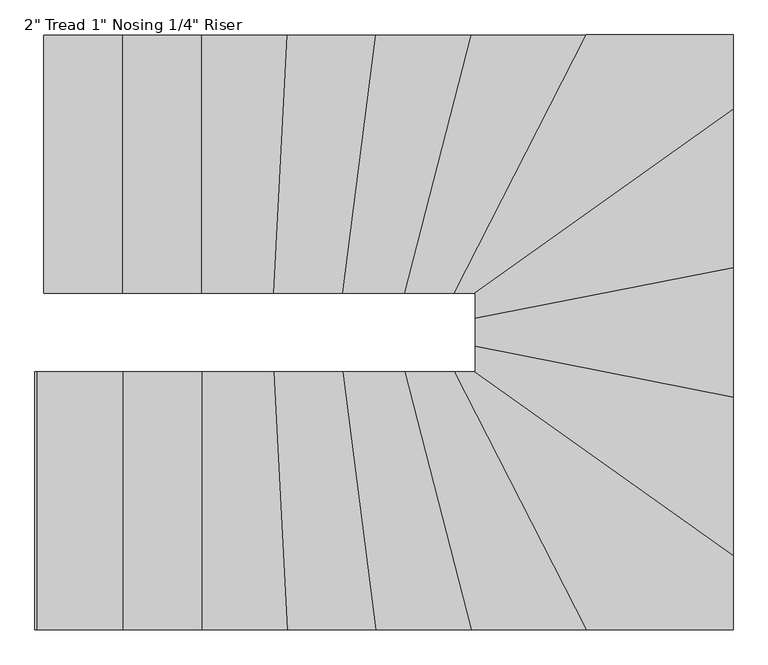
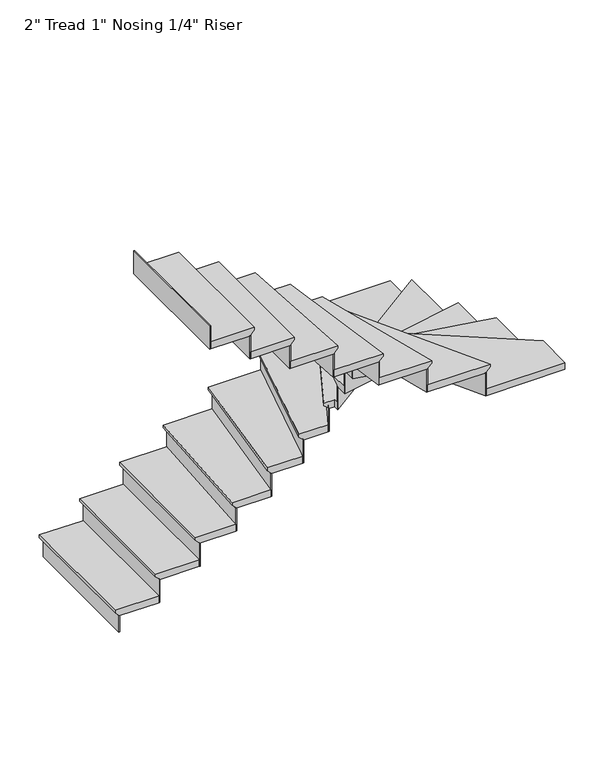
"""IFC4 building model written with IfcOpenShell, lengths in millimetres: stair flight geometry."""

from ifc_helpers import new_model, si_unit, origin, place, context, project, spatial, faceted_brep, source, transform, mapped, element, save


def stair_flight_58f01264(model_context):
    return source(origin(), model_context, "Body", "Brep", [
        faceted_brep([(-1451.7125891, 4613.9716937, 150.2833333), (-1451.7125891, 4613.9716937, 169.3333333), (-1451.7125891, 5528.3716937, 169.3333333), (-1451.7125891, 5528.3716937, 150.2833333), (-1426.3125891, 4613.9716937, 124.8833333), (-1426.3125891, 5528.3716937, 124.8833333), (-1146.9125891, 4613.9716937, 169.3333333), (-1146.9125891, 5528.3716937, 169.3333333), (-1426.3125891, 5528.3716937, 118.5333333), (-1146.9125891, 5528.3716937, 118.5333333), (-1146.9125891, 4613.9716937, 118.5333333), (-1426.3125891, 4613.9716937, 118.5333333)], [[[0, 1, 2, 3]], [[4, 0, 3, 5]], [[2, 1, 6, 7]], [[8, 9, 10, 11]], [[2, 7, 9, 8, 5, 3]], [[8, 11, 4, 5]], [[6, 1, 0, 4, 11, 10]], [[7, 6, 10, 9]]]),
        faceted_brep([(-1426.3125891, 4613.9716937, 118.5333333), (-1426.3125891, 4613.9716937, 0.0), (-1419.9625891, 4613.9716937, 0.0), (-1419.9625891, 4613.9716937, 118.5333333), (-1426.3125891, 5528.3716937, 118.5333333), (-1419.9625891, 5528.3716937, 118.5333333), (-1419.9625891, 5528.3716937, 0.0), (-1426.3125891, 5528.3716937, 0.0)], [[[0, 1, 2, 3]], [[4, 5, 6, 7]], [[1, 0, 4, 7]], [[2, 1, 7, 6]], [[3, 2, 6, 5]], [[0, 3, 5, 4]]]),
        faceted_brep([(-1146.9125891, 4613.9716937, 287.8666667), (-1146.9125891, 4613.9716937, 118.5333333), (-1140.5625891, 4613.9716937, 118.5333333), (-1140.5625891, 4613.9716937, 287.8666667), (-1146.9125891, 5528.3716937, 287.8666667), (-1140.5625891, 5528.3716937, 287.8666667), (-1140.5625891, 5528.3716937, 118.5333333), (-1146.9125891, 5528.3716937, 118.5333333)], [[[0, 1, 2, 3]], [[4, 5, 6, 7]], [[1, 0, 4, 7]], [[2, 1, 7, 6]], [[3, 2, 6, 5]], [[0, 3, 5, 4]]]),
        faceted_brep([(-1172.3125891, 5528.3716937, 338.6666667), (-1172.3125891, 4613.9716937, 338.6666667), (-867.5125891, 4613.9716937, 338.6666667), (-867.5125891, 5528.3716937, 338.6666667), (-1146.9125891, 5528.3716937, 287.8666667), (-867.5125891, 5528.3716937, 287.8666667), (-867.5125891, 4613.9716937, 287.8666667), (-1146.9125891, 4613.9716937, 287.8666667), (-1146.9125891, 5528.3716937, 294.2166667), (-1172.3125891, 5528.3716937, 319.6166667), (-1146.9125891, 4613.9716937, 294.2166667), (-1172.3125891, 4613.9716937, 319.6166667)], [[[0, 1, 2, 3]], [[4, 5, 6, 7]], [[0, 3, 5, 4, 8, 9]], [[4, 7, 10, 8]], [[2, 1, 11, 10, 7, 6]], [[3, 2, 6, 5]], [[11, 1, 0, 9]], [[10, 11, 9, 8]]]),
        faceted_brep([(-867.5125891, 4613.9716937, 457.2), (-867.5125891, 4613.9716937, 287.8666667), (-861.1625891, 4613.9716937, 287.8666667), (-861.1625891, 4613.9716937, 457.2), (-867.5125891, 5528.3716937, 457.2), (-861.1625891, 5528.3716937, 457.2), (-861.1625891, 5528.3716937, 287.8666667), (-867.5125891, 5528.3716937, 287.8666667)], [[[0, 1, 2, 3]], [[4, 5, 6, 7]], [[1, 0, 4, 7]], [[2, 1, 7, 6]], [[3, 2, 6, 5]], [[0, 3, 5, 4]]]),
        faceted_brep([(-892.9125891, 5528.3716937, 508.0), (-892.9125891, 4613.9716937, 508.0), (-611.8454276, 4613.9716937, 508.0), (-564.3111572, 5528.3716937, 508.0), (-867.5125891, 5528.3716937, 457.2), (-564.3111572, 5528.3716937, 457.2), (-611.8454276, 4613.9716937, 457.2), (-867.5125891, 4613.9716937, 457.2), (-867.5125891, 5528.3716937, 463.55), (-892.9125891, 5528.3716937, 488.95), (-867.5125891, 4613.9716937, 463.55), (-892.9125891, 4613.9716937, 488.95)], [[[0, 1, 2, 3]], [[4, 5, 6, 7]], [[0, 3, 5, 4, 8, 9]], [[4, 7, 10, 8]], [[2, 1, 11, 10, 7, 6]], [[3, 2, 6, 5]], [[11, 1, 0, 9]], [[10, 11, 9, 8]]]),
        faceted_brep([(-611.8454276, 4613.9716937, 626.5333333), (-611.8454276, 4613.9716937, 457.2), (-605.4868534, 4613.9716937, 457.2), (-605.4868534, 4613.9716937, 626.5333333), (-564.3111572, 5528.3716937, 626.5333333), (-557.952583, 5528.3716937, 626.5333333), (-557.952583, 5528.3716937, 457.2), (-564.3111572, 5528.3716937, 457.2)], [[[0, 1, 2, 3]], [[4, 5, 6, 7]], [[1, 0, 4, 7]], [[2, 1, 7, 6]], [[3, 2, 6, 5]], [[0, 3, 5, 4]]]),
        faceted_brep([(-589.7454539, 5528.3716937, 677.3333333), (-637.2797243, 4613.9716937, 677.3333333), (-367.6787278, 4613.9716937, 677.3333333), (-249.3226761, 5528.3716937, 677.3333333), (-564.3111572, 5528.3716937, 626.5333333), (-249.3226761, 5528.3716937, 626.5333333), (-367.6787278, 4613.9716937, 626.5333333), (-611.8454276, 4613.9716937, 626.5333333), (-564.3111572, 5528.3716937, 632.8833333), (-589.7454539, 5528.3716937, 658.2833333), (-611.8454276, 4613.9716937, 632.8833333), (-637.2797243, 4613.9716937, 658.2833333)], [[[0, 1, 2, 3]], [[4, 5, 6, 7]], [[0, 3, 5, 4, 8, 9]], [[4, 7, 10, 8]], [[2, 1, 11, 10, 7, 6]], [[3, 2, 6, 5]], [[11, 1, 0, 9]], [[10, 11, 9, 8]]]),
        faceted_brep([(-367.6787278, 4613.9716937, 795.8666667), (-367.6787278, 4613.9716937, 626.5333333), (-361.275756, 4613.9716937, 626.5333333), (-361.275756, 4613.9716937, 795.8666667), (-249.3226761, 5528.3716937, 795.8666667), (-242.9197043, 5528.3716937, 795.8666667), (-242.9197043, 5528.3716937, 626.5333333), (-249.3226761, 5528.3716937, 626.5333333)], [[[0, 1, 2, 3]], [[4, 5, 6, 7]], [[1, 0, 4, 7]], [[2, 1, 7, 6]], [[3, 2, 6, 5]], [[0, 3, 5, 4]]]),
        faceted_brep([(-274.9345632, 5528.3716937, 846.6666667), (-393.2906149, 4613.9716937, 846.6666667), (-146.0515053, 4613.9716937, 846.6666667), (89.0789421, 5528.3716937, 846.6666667), (-249.3226761, 5528.3716937, 795.8666667), (89.0789421, 5528.3716937, 795.8666667), (-146.0515053, 4613.9716937, 795.8666667), (-367.6787278, 4613.9716937, 795.8666667), (-249.3226761, 5528.3716937, 802.2166667), (-274.9345632, 5528.3716937, 827.6166667), (-367.6787278, 4613.9716937, 802.2166667), (-393.2906149, 4613.9716937, 827.6166667)], [[[0, 1, 2, 3]], [[4, 5, 6, 7]], [[0, 3, 5, 4, 8, 9]], [[4, 7, 10, 8]], [[2, 1, 11, 10, 7, 6]], [[3, 2, 6, 5]], [[11, 1, 0, 9]], [[10, 11, 9, 8]]]),
        faceted_brep([(-146.0515053, 4613.9716937, 965.2), (-146.0515053, 4613.9716937, 795.8666667), (-139.4949284, 4613.9716937, 795.8666667), (-139.4949284, 4613.9716937, 965.2), (89.0789421, 5528.3716937, 965.2), (95.635519, 5528.3716937, 965.2), (95.635519, 5528.3716937, 795.8666667), (89.0789421, 5528.3716937, 795.8666667)], [[[0, 1, 2, 3]], [[4, 5, 6, 7]], [[1, 0, 4, 7]], [[2, 1, 7, 6]], [[3, 2, 6, 5]], [[0, 3, 5, 4]]]),
        faceted_brep([(62.8526346, 5528.3716937, 1016.0), (-172.2778128, 4613.9716937, 1016.0), (30.2951308, 4613.9716937, 1016.0), (499.1197521, 5528.3716937, 1016.0), (89.0789421, 5528.3716937, 965.2), (499.1197521, 5528.3716937, 965.2), (30.2951308, 4613.9716937, 965.2), (-146.0515053, 4613.9716937, 965.2), (89.0789421, 5528.3716937, 971.55), (62.8526346, 5528.3716937, 996.95), (-146.0515053, 4613.9716937, 971.55), (-172.2778128, 4613.9716937, 996.95)], [[[0, 1, 2, 3]], [[4, 5, 6, 7]], [[0, 3, 5, 4, 8, 9]], [[4, 7, 10, 8]], [[2, 1, 11, 10, 7, 6]], [[3, 2, 6, 5]], [[11, 1, 0, 9]], [[10, 11, 9, 8]]]),
        faceted_brep([(30.2951308, 4613.9716937, 1134.5333333), (30.2951308, 4613.9716937, 965.2), (37.4311139, 4613.9716937, 965.2), (37.4311139, 4613.9716937, 1134.5333333), (499.1197521, 5528.3716937, 1134.5333333), (506.2557352, 5528.3716937, 1134.5333333), (506.2557352, 5528.3716937, 965.2), (499.1197521, 5528.3716937, 965.2)], [[[0, 1, 2, 3]], [[4, 5, 6, 7]], [[1, 0, 4, 7]], [[2, 1, 7, 6]], [[3, 2, 6, 5]], [[0, 3, 5, 4]]]),
        faceted_brep([(990.4191028, 5234.69056, 1185.3333333), (990.4191028, 5528.3716937, 1185.3333333), (470.5758196, 5528.3716937, 1185.3333333), (1.7511982, 4613.9716937, 1185.3333333), (76.0191028, 4613.9716937, 1185.3333333), (76.0191028, 4584.4166109, 1185.3333333), (990.4191028, 5528.3716937, 1134.5333333), (990.4191028, 5234.69056, 1134.5333333), (76.0191028, 4584.4166109, 1134.5333333), (76.0191028, 4613.9716937, 1134.5333333), (30.2951308, 4613.9716937, 1134.5333333), (499.1197521, 5528.3716937, 1134.5333333), (499.1197521, 5528.3716937, 1140.8833333), (470.5758196, 5528.3716937, 1166.2833333), (30.2951308, 4613.9716937, 1140.8833333), (1.7511982, 4613.9716937, 1166.2833333)], [[[0, 1, 2, 3, 4, 5]], [[6, 7, 8, 9, 10, 11]], [[1, 0, 7, 6]], [[2, 1, 6, 11, 12, 13]], [[11, 10, 14, 12]], [[4, 3, 15, 14, 10, 9]], [[5, 4, 9, 8]], [[0, 5, 8, 7]], [[15, 3, 2, 13]], [[14, 15, 13, 12]]]),
        faceted_brep([(76.0191028, 4584.4166109, 1303.8666667), (76.0191028, 4584.4166109, 1134.5333333), (76.0191028, 4576.6246361, 1134.5333333), (76.0191028, 4576.6246361, 1303.8666667), (990.4191028, 5234.69056, 1303.8666667), (990.4191028, 5226.8985852, 1303.8666667), (990.4191028, 5226.8985852, 1134.5333333), (990.4191028, 5234.69056, 1134.5333333)], [[[0, 1, 2, 3]], [[4, 5, 6, 7]], [[1, 0, 4, 7]], [[2, 1, 7, 6]], [[3, 2, 6, 5]], [[0, 3, 5, 4]]]),
        faceted_brep([(990.4191028, 5265.8584592, 1354.6666667), (76.0191028, 4615.58451, 1354.6666667), (76.0191028, 4497.9625238, 1354.6666667), (990.4191028, 4678.2033801, 1354.6666667), (990.4191028, 5234.69056, 1303.8666667), (990.4191028, 4678.2033801, 1303.8666667), (76.0191028, 4497.9625238, 1303.8666667), (76.0191028, 4584.4166109, 1303.8666667), (990.4191028, 5234.69056, 1310.2166667), (990.4191028, 5265.8584592, 1335.6166667), (76.0191028, 4584.4166109, 1310.2166667), (76.0191028, 4615.58451, 1335.6166667)], [[[0, 1, 2, 3]], [[4, 5, 6, 7]], [[0, 3, 5, 4, 8, 9]], [[4, 7, 10, 8]], [[2, 1, 11, 10, 7, 6]], [[3, 2, 6, 5]], [[11, 1, 0, 9]], [[10, 11, 9, 8]]]),
        faceted_brep([(76.0191028, 4497.9625238, 1473.2), (76.0191028, 4497.9625238, 1303.8666667), (76.0191028, 4491.4903384, 1303.8666667), (76.0191028, 4491.4903384, 1473.2), (990.4191028, 4678.2033801, 1473.2), (990.4191028, 4671.7311947, 1473.2), (990.4191028, 4671.7311947, 1303.8666667), (990.4191028, 4678.2033801, 1303.8666667)], [[[0, 1, 2, 3]], [[4, 5, 6, 7]], [[1, 0, 4, 7]], [[2, 1, 7, 6]], [[3, 2, 6, 5]], [[0, 3, 5, 4]]]),
        faceted_brep([(990.4191028, 4704.0921219, 1524.0), (76.0191028, 4523.8512655, 1524.0), (76.0191028, 4398.8033801, 1524.0), (990.4191028, 4218.5625238, 1524.0), (990.4191028, 4678.2033801, 1473.2), (990.4191028, 4218.5625238, 1473.2), (76.0191028, 4398.8033801, 1473.2), (76.0191028, 4497.9625238, 1473.2), (990.4191028, 4678.2033801, 1479.55), (990.4191028, 4704.0921219, 1504.95), (76.0191028, 4497.9625238, 1479.55), (76.0191028, 4523.8512655, 1504.95)], [[[0, 1, 2, 3]], [[4, 5, 6, 7]], [[0, 3, 5, 4, 8, 9]], [[4, 7, 10, 8]], [[2, 1, 11, 10, 7, 6]], [[3, 2, 6, 5]], [[11, 1, 0, 9]], [[10, 11, 9, 8]]]),
        faceted_brep([(76.0191028, 4398.8033801, 1642.5333333), (76.0191028, 4398.8033801, 1473.2), (76.0191028, 4392.3311947, 1473.2), (76.0191028, 4392.3311947, 1642.5333333), (990.4191028, 4218.5625238, 1642.5333333), (990.4191028, 4212.0903384, 1642.5333333), (990.4191028, 4212.0903384, 1473.2), (990.4191028, 4218.5625238, 1473.2)], [[[0, 1, 2, 3]], [[4, 5, 6, 7]], [[1, 0, 4, 7]], [[2, 1, 7, 6]], [[3, 2, 6, 5]], [[0, 3, 5, 4]]]),
        faceted_brep([(990.4191028, 4244.4512655, 1693.3333333), (76.0191028, 4424.6921219, 1693.3333333), (76.0191028, 4334.5716937, 1693.3333333), (29.9236283, 4334.5716937, 1693.3333333), (990.4191028, 3651.517029, 1693.3333333), (990.4191028, 4218.5625238, 1642.5333333), (990.4191028, 3651.517029, 1642.5333333), (29.9236283, 4334.5716937, 1642.5333333), (76.0191028, 4334.5716937, 1642.5333333), (76.0191028, 4398.8033801, 1642.5333333), (990.4191028, 4218.5625238, 1648.8833333), (990.4191028, 4244.4512655, 1674.2833333), (76.0191028, 4398.8033801, 1648.8833333), (76.0191028, 4424.6921219, 1674.2833333)], [[[0, 1, 2, 3, 4]], [[5, 6, 7, 8, 9]], [[0, 4, 6, 5, 10, 11]], [[5, 9, 12, 10]], [[2, 1, 13, 12, 9, 8]], [[3, 2, 8, 7]], [[4, 3, 7, 6]], [[13, 1, 0, 11]], [[12, 13, 11, 10]]]),
        faceted_brep([(29.9236283, 4334.5716937, 1811.8666667), (29.9236283, 4334.5716937, 1642.5333333), (18.9667358, 4334.5716937, 1642.5333333), (18.9667358, 4334.5716937, 1811.8666667), (990.4191028, 3651.517029, 1811.8666667), (990.4191028, 3643.7250543, 1811.8666667), (990.4191028, 3643.7250543, 1642.5333333), (990.4191028, 3651.517029, 1642.5333333)], [[[0, 1, 2, 3]], [[4, 5, 6, 7]], [[1, 0, 4, 7]], [[2, 1, 7, 6]], [[3, 2, 6, 5]], [[0, 3, 5, 4]]]),
        faceted_brep([(442.031887, 3420.1716937, 1862.6666667), (990.4191028, 3420.1716937, 1862.6666667), (990.4191028, 3682.6849282, 1862.6666667), (73.7511982, 4334.5716937, 1862.6666667), (-26.7927343, 4334.5716937, 1862.6666667), (990.4191028, 3420.1716937, 1811.8666667), (442.031887, 3420.1716937, 1811.8666667), (-26.7927343, 4334.5716937, 1811.8666667), (29.9236283, 4334.5716937, 1811.8666667), (990.4191028, 3651.517029, 1811.8666667), (990.4191028, 3651.517029, 1818.2166667), (990.4191028, 3682.6849282, 1843.6166667), (29.9236283, 4334.5716937, 1818.2166667), (73.7511982, 4334.5716937, 1843.6166667)], [[[0, 1, 2, 3, 4]], [[5, 6, 7, 8, 9]], [[1, 0, 6, 5]], [[2, 1, 5, 9, 10, 11]], [[9, 8, 12, 10]], [[4, 3, 13, 12, 8, 7]], [[0, 4, 7, 6]], [[13, 3, 2, 11]], [[12, 13, 11, 10]]]),
        faceted_brep([(-26.7927343, 4334.5716937, 1981.2), (-26.7927343, 4334.5716937, 1811.8666667), (-33.9287174, 4334.5716937, 1811.8666667), (-33.9287174, 4334.5716937, 1981.2), (442.031887, 3420.1716937, 1981.2), (434.8959039, 3420.1716937, 1981.2), (434.8959039, 3420.1716937, 1811.8666667), (442.031887, 3420.1716937, 1811.8666667)], [[[0, 1, 2, 3]], [[4, 5, 6, 7]], [[1, 0, 4, 7]], [[2, 1, 7, 6]], [[3, 2, 6, 5]], [[0, 3, 5, 4]]]),
        faceted_brep([(470.5758196, 3420.1716937, 2032.0), (1.7511982, 4334.5716937, 2032.0), (-198.5041202, 4334.5716937, 2032.0), (36.6263272, 3420.1716937, 2032.0), (442.031887, 3420.1716937, 1981.2), (36.6263272, 3420.1716937, 1981.2), (-198.5041202, 4334.5716937, 1981.2), (-26.7927343, 4334.5716937, 1981.2), (442.031887, 3420.1716937, 1987.55), (470.5758196, 3420.1716937, 2012.95), (-26.7927343, 4334.5716937, 1987.55), (1.7511982, 4334.5716937, 2012.95)], [[[0, 1, 2, 3]], [[4, 5, 6, 7]], [[0, 3, 5, 4, 8, 9]], [[4, 7, 10, 8]], [[2, 1, 11, 10, 7, 6]], [[3, 2, 6, 5]], [[11, 1, 0, 9]], [[10, 11, 9, 8]]]),
        faceted_brep([(-198.5041202, 4334.5716937, 2150.5333333), (-198.5041202, 4334.5716937, 1981.2), (-205.0606971, 4334.5716937, 1981.2), (-205.0606971, 4334.5716937, 2150.5333333), (36.6263272, 3420.1716937, 2150.5333333), (30.0697503, 3420.1716937, 2150.5333333), (30.0697503, 3420.1716937, 1981.2), (36.6263272, 3420.1716937, 1981.2)], [[[0, 1, 2, 3]], [[4, 5, 6, 7]], [[1, 0, 4, 7]], [[2, 1, 7, 6]], [[3, 2, 6, 5]], [[0, 3, 5, 4]]]),
        faceted_brep([(62.8526346, 3420.1716937, 2201.3333333), (-172.2778128, 4334.5716937, 2201.3333333), (-418.902502, 4334.5716937, 2201.3333333), (-300.5464504, 3420.1716937, 2201.3333333), (36.6263272, 3420.1716937, 2150.5333333), (-300.5464504, 3420.1716937, 2150.5333333), (-418.902502, 4334.5716937, 2150.5333333), (-198.5041202, 4334.5716937, 2150.5333333), (36.6263272, 3420.1716937, 2156.8833333), (62.8526346, 3420.1716937, 2182.2833333), (-198.5041202, 4334.5716937, 2156.8833333), (-172.2778128, 4334.5716937, 2182.2833333)], [[[0, 1, 2, 3]], [[4, 5, 6, 7]], [[0, 3, 5, 4, 8, 9]], [[4, 7, 10, 8]], [[2, 1, 11, 10, 7, 6]], [[3, 2, 6, 5]], [[11, 1, 0, 9]], [[10, 11, 9, 8]]]),
        faceted_brep([(-418.902502, 4334.5716937, 2319.8666667), (-418.902502, 4334.5716937, 2150.5333333), (-425.3054738, 4334.5716937, 2150.5333333), (-425.3054738, 4334.5716937, 2319.8666667), (-300.5464504, 3420.1716937, 2319.8666667), (-306.9494221, 3420.1716937, 2319.8666667), (-306.9494221, 3420.1716937, 2150.5333333), (-300.5464504, 3420.1716937, 2150.5333333)], [[[0, 1, 2, 3]], [[4, 5, 6, 7]], [[1, 0, 4, 7]], [[2, 1, 7, 6]], [[3, 2, 6, 5]], [[0, 3, 5, 4]]]),
        faceted_brep([(-274.9345632, 3420.1716937, 2370.6666667), (-393.2906149, 4334.5716937, 2370.6666667), (-662.7140209, 4334.5716937, 2370.6666667), (-615.1797505, 3420.1716937, 2370.6666667), (-300.5464504, 3420.1716937, 2319.8666667), (-615.1797505, 3420.1716937, 2319.8666667), (-662.7140209, 4334.5716937, 2319.8666667), (-418.902502, 4334.5716937, 2319.8666667), (-300.5464504, 3420.1716937, 2326.2166667), (-274.9345632, 3420.1716937, 2351.6166667), (-418.902502, 4334.5716937, 2326.2166667), (-393.2906149, 4334.5716937, 2351.6166667)], [[[0, 1, 2, 3]], [[4, 5, 6, 7]], [[0, 3, 5, 4, 8, 9]], [[4, 7, 10, 8]], [[2, 1, 11, 10, 7, 6]], [[3, 2, 6, 5]], [[11, 1, 0, 9]], [[10, 11, 9, 8]]]),
        faceted_brep([(-662.7140209, 4334.5716937, 2489.2), (-662.7140209, 4334.5716937, 2319.8666667), (-669.0725951, 4334.5716937, 2319.8666667), (-669.0725951, 4334.5716937, 2489.2), (-615.1797505, 3420.1716937, 2489.2), (-621.5383247, 3420.1716937, 2489.2), (-621.5383247, 3420.1716937, 2319.8666667), (-615.1797505, 3420.1716937, 2319.8666667)], [[[0, 1, 2, 3]], [[4, 5, 6, 7]], [[1, 0, 4, 7]], [[2, 1, 7, 6]], [[3, 2, 6, 5]], [[0, 3, 5, 4]]]),
        faceted_brep([(-589.7454539, 3420.1716937, 2540.0), (-637.2797243, 4334.5716937, 2540.0), (-918.3125891, 4334.5716937, 2540.0), (-918.3125891, 3420.1716937, 2540.0), (-615.1797505, 3420.1716937, 2489.2), (-918.3125891, 3420.1716937, 2489.2), (-918.3125891, 4334.5716937, 2489.2), (-662.7140209, 4334.5716937, 2489.2), (-615.1797505, 3420.1716937, 2495.55), (-589.7454539, 3420.1716937, 2520.95), (-662.7140209, 4334.5716937, 2495.55), (-637.2797243, 4334.5716937, 2520.95)], [[[0, 1, 2, 3]], [[4, 5, 6, 7]], [[0, 3, 5, 4, 8, 9]], [[4, 7, 10, 8]], [[2, 1, 11, 10, 7, 6]], [[3, 2, 6, 5]], [[11, 1, 0, 9]], [[10, 11, 9, 8]]]),
        faceted_brep([(-918.3125891, 4334.5716937, 2658.5333333), (-918.3125891, 4334.5716937, 2489.2), (-924.6625891, 4334.5716937, 2489.2), (-924.6625891, 4334.5716937, 2658.5333333), (-918.3125891, 3420.1716937, 2658.5333333), (-924.6625891, 3420.1716937, 2658.5333333), (-924.6625891, 3420.1716937, 2489.2), (-918.3125891, 3420.1716937, 2489.2)], [[[0, 1, 2, 3]], [[4, 5, 6, 7]], [[1, 0, 4, 7]], [[2, 1, 7, 6]], [[3, 2, 6, 5]], [[0, 3, 5, 4]]]),
        faceted_brep([(-892.9125891, 3420.1716937, 2709.3333333), (-892.9125891, 4334.5716937, 2709.3333333), (-1197.7125891, 4334.5716937, 2709.3333333), (-1197.7125891, 3420.1716937, 2709.3333333), (-918.3125891, 3420.1716937, 2658.5333333), (-1197.7125891, 3420.1716937, 2658.5333333), (-1197.7125891, 4334.5716937, 2658.5333333), (-918.3125891, 4334.5716937, 2658.5333333), (-918.3125891, 3420.1716937, 2664.8833333), (-892.9125891, 3420.1716937, 2690.2833333), (-918.3125891, 4334.5716937, 2664.8833333), (-892.9125891, 4334.5716937, 2690.2833333)], [[[0, 1, 2, 3]], [[4, 5, 6, 7]], [[0, 3, 5, 4, 8, 9]], [[4, 7, 10, 8]], [[2, 1, 11, 10, 7, 6]], [[3, 2, 6, 5]], [[11, 1, 0, 9]], [[10, 11, 9, 8]]]),
        faceted_brep([(-1197.7125891, 4334.5716937, 2827.8666667), (-1197.7125891, 4334.5716937, 2658.5333333), (-1204.0625891, 4334.5716937, 2658.5333333), (-1204.0625891, 4334.5716937, 2827.8666667), (-1197.7125891, 3420.1716937, 2827.8666667), (-1204.0625891, 3420.1716937, 2827.8666667), (-1204.0625891, 3420.1716937, 2658.5333333), (-1197.7125891, 3420.1716937, 2658.5333333)], [[[0, 1, 2, 3]], [[4, 5, 6, 7]], [[1, 0, 4, 7]], [[2, 1, 7, 6]], [[3, 2, 6, 5]], [[0, 3, 5, 4]]]),
        faceted_brep([(-1477.1125891, 4334.5716937, 2997.2), (-1477.1125891, 4334.5716937, 2827.8666667), (-1483.4625891, 4334.5716937, 2827.8666667), (-1483.4625891, 4334.5716937, 2997.2), (-1477.1125891, 3420.1716937, 2997.2), (-1483.4625891, 3420.1716937, 2997.2), (-1483.4625891, 3420.1716937, 2827.8666667), (-1477.1125891, 3420.1716937, 2827.8666667)], [[[0, 1, 2, 3]], [[4, 5, 6, 7]], [[1, 0, 4, 7]], [[2, 1, 7, 6]], [[3, 2, 6, 5]], [[0, 3, 5, 4]]]),
        faceted_brep([(-1172.3125891, 3420.1716937, 2878.6666667), (-1172.3125891, 4334.5716937, 2878.6666667), (-1477.1125891, 4334.5716937, 2878.6666667), (-1477.1125891, 3420.1716937, 2878.6666667), (-1197.7125891, 3420.1716937, 2827.8666667), (-1477.1125891, 3420.1716937, 2827.8666667), (-1477.1125891, 4334.5716937, 2827.8666667), (-1197.7125891, 4334.5716937, 2827.8666667), (-1197.7125891, 3420.1716937, 2834.2166667), (-1172.3125891, 3420.1716937, 2859.6166667), (-1197.7125891, 4334.5716937, 2834.2166667), (-1172.3125891, 4334.5716937, 2859.6166667)], [[[0, 1, 2, 3]], [[4, 5, 6, 7]], [[0, 3, 5, 4, 8, 9]], [[4, 7, 10, 8]], [[2, 1, 11, 10, 7, 6]], [[3, 2, 6, 5]], [[11, 1, 0, 9]], [[10, 11, 9, 8]]]),
    ])


if __name__ == "__main__":
    model = new_model("IFC4")
    model_context = context("Model", 3, world=origin())
    ifc_project = project(units=[si_unit("LENGTHUNIT", "METRE", prefix="MILLI")], contexts=[model_context])
    site = spatial("IfcSite", under=ifc_project)
    building = spatial("IfcBuilding", under=site)
    placement = place(None, origin())
    stair_flight_shape = stair_flight_58f01264(model_context)
    element("IfcStairFlight", 1, ObjectType="2\" Tread 1\" Nosing 1/4\" Riser", at=placement, inside=building, context=model_context, shape_type="MappedRepresentation", body=[
        mapped(stair_flight_shape, transform((0.0, 0.0, 0.0), x_axis=(1.0, 0.0, 0.0), y_axis=(0.0, 1.0, 0.0), z_axis=(0.0, 0.0, 1.0))),
    ])
    save(model, "model.ifc")
